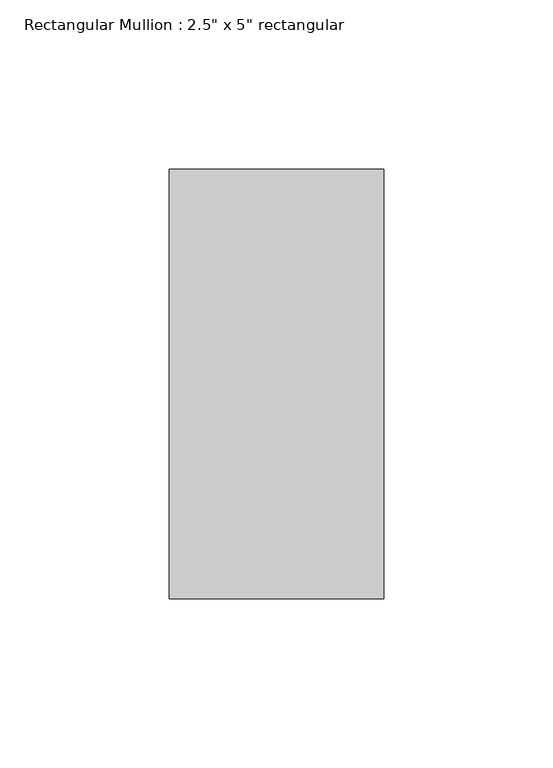
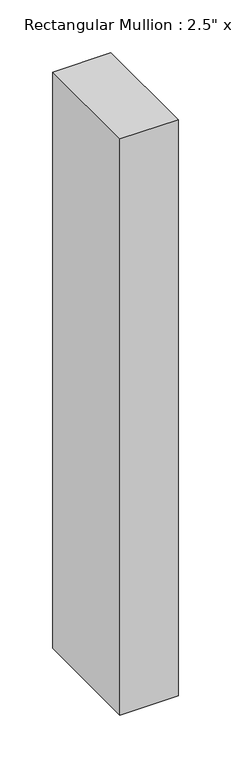
"""IFC4 building model written with IfcOpenShell, lengths in millimetres: member geometry."""

from ifc_helpers import new_model, si_unit, frame, origin, place, context, project, spatial, polyline, outline, extrude, source, transform, mapped, element, save


def member_418a0375(model_context):
    return source(origin(), model_context, "Body", "SweptSolid", [
        extrude(outline(polyline([(0.0, 63.5), (0.0, -63.5), (-63.5, -63.5), (-63.5, 63.5), (0.0, 63.5)])), frame((0.0, 0.0, -665.5842307), z_axis=(0.0, 0.0, 1.0), x_axis=(1.0, 0.0, 0.0)), (0.0, 0.0, 1.0), 665.5842307),
    ])


if __name__ == "__main__":
    model = new_model("IFC4")
    model_context = context("Model", 3, world=origin())
    ifc_project = project(units=[si_unit("LENGTHUNIT", "METRE", prefix="MILLI")], contexts=[model_context])
    site = spatial("IfcSite", under=ifc_project)
    building = spatial("IfcBuilding", under=site)
    placement = place(None, origin())
    member_shape = member_418a0375(model_context)
    element("IfcMember", 1, ObjectType="Rectangular Mullion : 2.5\" x 5\" rectangular", at=placement, inside=building, context=model_context, shape_type="MappedRepresentation", body=[
        mapped(member_shape, transform((0.0, 0.0, 0.0), x_axis=(1.0, 0.0, 0.0), y_axis=(0.0, 1.0, 0.0), z_axis=(0.0, 0.0, 1.0))),
    ])
    save(model, "model.ifc")

# Revit data of these elements
# Type "Rectangular Mullion : 2.5\" x 5\" rectangular"
#   built-in parameter 1007304 = 0.416667 (stored number, unit not read)
#   built-in parameter 1007301 = 0.104167 (stored number, unit not read)
#   built-in parameter 1007300 = 0.104167 (stored number, unit not read)
# Element 1 (IfcMember, "Rectangular Mullion : 2.5\" x 5\" rectangular")
#   Materials on its faces: "Aluminum"
# Materials
#   "Aluminum": class "Metal", colour RGB 247 247 247, transparency 0, Description = "Aluminum 6061", Cost = 0
